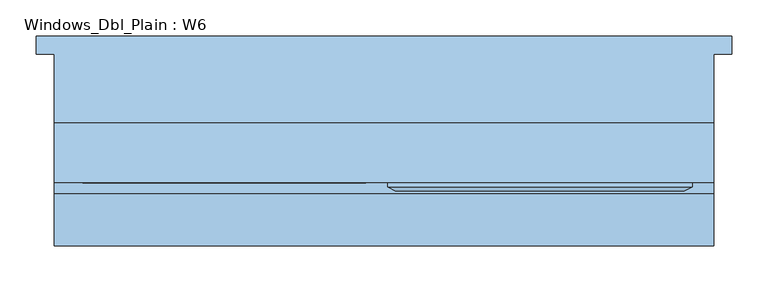
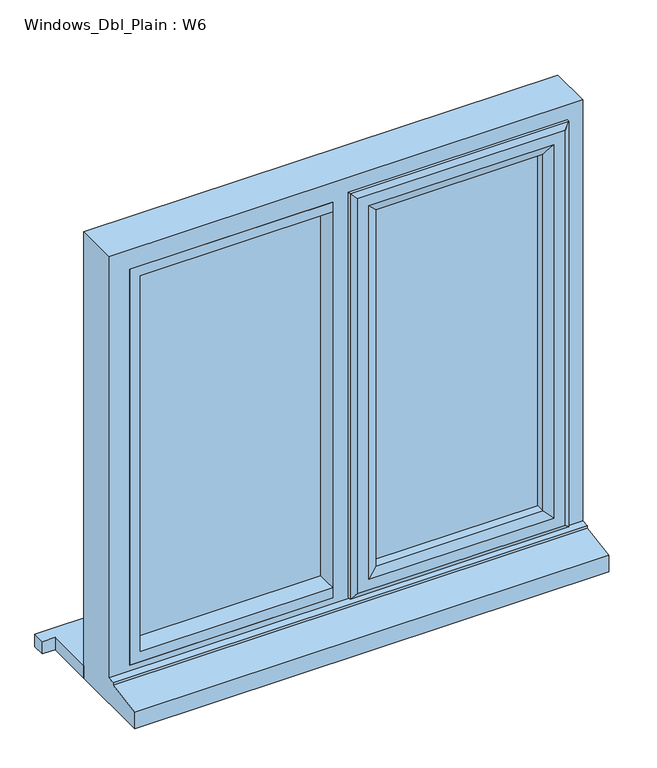
"""IFC4 building model written with IfcOpenShell, lengths in millimetres: window geometry, Windows_Dbl_Plain : W6."""

from ifc_helpers import new_model, si_unit, frame, origin, place, context, project, spatial, polyline, outline, extrude, faceted_brep, source, transform, mapped, element, save


def windows_dbl_plain_w6_14064f4c(model_context):
    return source(origin(), model_context, "Body", "SolidModel", [
        extrude(outline(polyline([(-767.2, 130.8434322), (197.2, 130.8434322), (197.2, 105.8434322), (172.2, 105.8434322), (172.2, 10.2434322), (-742.2, 10.2434322), (-742.2, 105.8434322), (-767.2, 105.8434322), (-767.2, 130.8434322)])), frame((0.0, 0.0, 1200.0), z_axis=(0.0, 0.0, 1.0), x_axis=(1.0, 0.0, 0.0)), (0.0, 0.0, 1.0), 25.0),
        faceted_brep([(-280.0, -72.7565678, 2080.0), (-280.0, -72.7565678, 1253.0), (-280.0, -78.5300705, 1253.0), (-280.0, -78.5300705, 2080.0), (-270.0, -7.7565678, 2070.0), (-270.0, -7.7565678, 1263.0), (-270.0, -72.7565678, 1263.0), (-270.0, -72.7565678, 2070.0), (-230.0, -22.2494677, 2030.0), (-230.0, -22.2494677, 1303.0), (-240.1480377, -7.7565678, 1292.8519623), (-240.1480377, -7.7565678, 2040.1480377), (-230.0, -36.7565678, 2030.0), (-230.0, -36.7565678, 1303.0), (-240.0, -60.7565678, 2040.0), (-240.0, -60.7565678, 1293.0), (-240.0, -36.7565678, 1293.0), (-240.0, -36.7565678, 2040.0), (-230.0, -78.5300705, 2030.0), (-230.0, -78.5300705, 1303.0), (-230.0, -60.7565678, 1303.0), (-230.0, -60.7565678, 2030.0), (-247.4457548, -84.3035732, 2047.4457548), (-247.4457548, -84.3035732, 1285.5542452), (-269.2153903, -84.3035732, 1263.7846097), (-269.2153903, -84.3035732, 2069.2153903), (142.2, -72.7565678, 1253.0), (142.2, -78.5300705, 1253.0), (132.2, -7.7565678, 1263.0), (132.2, -72.7565678, 1263.0), (92.2, -22.2494677, 1303.0), (102.3480377, -7.7565678, 1292.8519623), (92.2, -36.7565678, 1303.0), (102.2, -60.7565678, 1293.0), (102.2, -36.7565678, 1293.0), (92.2, -78.5300705, 1303.0), (92.2, -60.7565678, 1303.0), (109.6457548, -84.3035732, 1285.5542452), (131.4153903, -84.3035732, 1263.7846097), (142.2, -72.7565678, 2080.0), (142.2, -78.5300705, 2080.0), (132.2, -7.7565678, 2070.0), (132.2, -72.7565678, 2070.0), (92.2, -22.2494677, 2030.0), (102.3480377, -7.7565678, 2040.1480377), (92.2, -36.7565678, 2030.0), (102.2, -60.7565678, 2040.0), (102.2, -36.7565678, 2040.0), (92.2, -78.5300705, 2030.0), (92.2, -60.7565678, 2030.0), (109.6457548, -84.3035732, 2047.4457548), (131.4153903, -84.3035732, 2069.2153903)], [[[0, 1, 2, 3]], [[4, 5, 6, 7]], [[8, 9, 10, 11]], [[12, 13, 9, 8]], [[14, 15, 16, 17]], [[18, 19, 20, 21]], [[22, 23, 19, 18]], [[3, 2, 24, 25]], [[1, 26, 27, 2]], [[5, 28, 29, 6]], [[9, 30, 31, 10]], [[13, 32, 30, 9]], [[15, 33, 34, 16]], [[19, 35, 36, 20]], [[23, 37, 35, 19]], [[2, 27, 38, 24]], [[26, 39, 40, 27]], [[28, 41, 42, 29]], [[30, 43, 44, 31]], [[32, 45, 43, 30]], [[33, 46, 47, 34]], [[35, 48, 49, 36]], [[37, 50, 48, 35]], [[27, 40, 51, 38]], [[39, 0, 3, 40]], [[1, 0, 39, 26], [7, 6, 29, 42]], [[41, 4, 7, 42]], [[5, 4, 41, 28], [11, 10, 31, 44]], [[43, 8, 11, 44]], [[45, 12, 8, 43]], [[17, 16, 34, 47], [13, 12, 45, 32]], [[46, 14, 17, 47]], [[15, 14, 46, 33], [21, 20, 36, 49]], [[48, 18, 21, 49]], [[50, 22, 18, 48]], [[25, 24, 38, 51], [23, 22, 50, 37]], [[40, 3, 25, 51]]]),
        extrude(outline(polyline([(2070.0, -310.0), (2070.0, -702.2), (1263.0, -702.2), (1263.0, -310.0), (1283.0, -310.0), (1283.0, -682.2), (2050.0, -682.2), (2050.0, -310.0), (2070.0, -310.0)])), frame((0.0, -72.7565678, 0.0), z_axis=(0.0, 1.0, 0.0), x_axis=(0.0, 0.0, 1.0)), (0.0, 0.0, 1.0), 41.0),
        faceted_brep([(172.2, 10.2434322, 2110.0), (172.2, 10.2434322, 1200.0), (-742.2, 10.2434322, 1200.0), (-742.2, 10.2434322, 2110.0), (112.2, 10.2434322, 2050.0), (-252.0, 10.2434322, 2050.0), (-252.0, 10.2434322, 1275.0), (112.2, 10.2434322, 1275.0), (-310.0, 10.2434322, 2050.0), (-682.2, 10.2434322, 2050.0), (-682.2, 10.2434322, 1275.0), (-310.0, 10.2434322, 1275.0), (-742.2, -160.2565678, 1200.0), (-742.2, -160.2565678, 1233.8088847), (-742.2, -87.7565678, 1244.7449676), (-742.2, -87.7565678, 1249.68767), (-742.2, -72.7565678, 1251.0), (-742.2, -72.7565678, 2110.0), (172.2, -72.7565678, 1251.0), (172.2, -72.7565678, 2110.0), (-702.2, -72.7565678, 2070.0), (-310.0, -72.7565678, 2070.0), (-310.0, -72.7565678, 1263.0), (-702.2, -72.7565678, 1263.0), (-270.0, -72.7565678, 2070.0), (132.2, -72.7565678, 2070.0), (132.2, -72.7565678, 1263.0), (-270.0, -72.7565678, 1263.0), (-702.2, -7.7565678, 1263.0), (-702.2, -7.7565678, 2070.0), (-300.0, -7.7565678, 1263.0), (-300.0, -7.7565678, 2070.0), (-310.0, -7.7565678, 2050.0), (-310.0, -7.7565678, 1275.0), (-682.2, -7.7565678, 1275.0), (-682.2, -7.7565678, 2050.0), (-270.0, -7.7565678, 2070.0), (-270.0, -7.7565678, 1263.0), (132.2, -7.7565678, 1263.0), (132.2, -7.7565678, 2070.0), (112.2, -7.7565678, 2050.0), (112.2, -7.7565678, 1275.0), (-252.0, -7.7565678, 1275.0), (-252.0, -7.7565678, 2050.0), (-300.0, -31.7565678, 2070.0), (-310.0, -31.7565678, 2070.0), (172.2, -87.7565678, 1249.68767), (172.2, -87.7565678, 1244.7449676), (172.2, -160.2565678, 1233.8088847), (172.2, -160.2565678, 1200.0), (-300.0, -31.7565678, 1263.0), (-310.0, -31.7565678, 1263.0)], [[[0, 1, 2, 3], [4, 5, 6, 7], [8, 9, 10, 11]], [[2, 12, 13, 14, 15, 16, 17, 3]], [[16, 18, 19, 17], [20, 21, 22, 23], [24, 25, 26, 27]], [[23, 28, 29, 20]], [[29, 28, 30, 31], [32, 33, 34, 35]], [[36, 37, 38, 39], [40, 41, 42, 43]], [[35, 34, 10, 9]], [[3, 17, 19, 0]], [[25, 24, 36, 39]], [[29, 31, 44, 45, 21, 20]], [[9, 8, 32, 35]], [[40, 43, 5, 4]], [[18, 46, 47, 48, 49, 1, 0, 19]], [[25, 39, 38, 26]], [[4, 7, 41, 40]], [[44, 31, 30, 50]], [[50, 51, 45, 44]], [[51, 22, 21, 45]], [[27, 37, 36, 24]], [[43, 42, 6, 5]], [[8, 11, 33, 32]], [[49, 12, 2, 1]], [[48, 13, 12, 49]], [[47, 14, 13, 48]], [[46, 15, 14, 47]], [[18, 16, 15, 46]], [[26, 38, 37, 27]], [[22, 51, 50, 30, 28, 23]], [[6, 42, 41, 7]], [[33, 11, 10, 34]]]),
        extrude(outline(polyline([(-702.2, -31.7565678), (-702.2, -7.7565678), (-300.0, -7.7565678), (-300.0, -31.7565678), (-702.2, -31.7565678)])), frame((0.0, 0.0, 1263.0), z_axis=(0.0, 0.0, 1.0), x_axis=(1.0, 0.0, 0.0)), (0.0, 0.0, 1.0), 807.0),
        extrude(outline(polyline([(102.2, -36.7565678), (102.2, -60.7565678), (-240.0, -60.7565678), (-240.0, -36.7565678), (102.2, -36.7565678)])), frame((0.0, 0.0, 1293.0), z_axis=(0.0, 0.0, 1.0), x_axis=(1.0, 0.0, 0.0)), (0.0, 0.0, 1.0), 747.0),
    ])


if __name__ == "__main__":
    model = new_model("IFC4")
    model_context = context("Model", 3, world=origin())
    ifc_project = project(units=[si_unit("LENGTHUNIT", "METRE", prefix="MILLI")], contexts=[model_context])
    site = spatial("IfcSite", under=ifc_project)
    building = spatial("IfcBuilding", under=site)
    placement = place(None, origin())
    windows_dbl_plain_w6_shape = windows_dbl_plain_w6_14064f4c(model_context)
    element("IfcWindow", 1, ObjectType="Windows_Dbl_Plain : W6", at=placement, inside=building, context=model_context, shape_type="MappedRepresentation", body=[
        mapped(windows_dbl_plain_w6_shape, transform((0.0, 0.0, 0.0), x_axis=(1.0, 0.0, 0.0), y_axis=(0.0, 1.0, 0.0), z_axis=(0.0, 0.0, 1.0))),
    ])
    save(model, "model.ifc")

# Revit data of these elements
# Type "Windows_Dbl_Plain : W6"
#   Type Mark = "56"
#   Operation = "DoublePanelVertical"
#   Construction Type Id = "GSP4R"
#   Manufacturer = "Revit"
#   Keynote = "L10"
#   Analytic Construction = "1/8 in Pilkington single glazing"
#   Wrap Layers (Ext) from Ext = 0.336286 ft
#   Wrap Layers (Int) from Ext = 0.582349 ft
#   Window Board Projection = 0.082021 ft
#   Window Board Extension = 0.082021 ft
#   Visual Light Transmittance = 0.9
#   Solar Heat Gain Coefficient = 0.78
#   Rough Width = 3.0 ft
#   Rough Height = 2.985564 ft
#   Height = 2.985564 ft
#   Width = 3.0 ft
#   Heat Transfer Coefficient (U) = 3.6886 W/(m²·K)
#   Glazing Thickness = 0.07874 ft
#   FrameOffset - External = 0.164042 ft
#   Frame Depth = 0.213255 ft
#   Default Head Height = 6.922572 ft
#   Cill Depth = 0.287073 ft
#   Cavity Closer Width = 0.164042 ft
#   Cavity Closer Offset from Ext = 0.336286 ft
#   Cavity Closer Depth = 0.278871 ft
#   Vis - Cavity Closers = yes
#   Define Thermal Properties by = 1
#   Material Trim = Window Frame
#   Material Glass = Glass
#   Material Frame = Cherry
#   Wall Closure = (empty or 0)
# Element 1 (IfcWindow, "Windows_Dbl_Plain : W6")
#   Materials on its faces: "Cherry", "Glass", "Window Frame"
# Materials
#   "Window Frame": colour RGB 249 249 249, transparency 0, Keynote = "L10", Cost = 0
#   "Glass": class "Glass", colour RGB 0 128 192, transparency 0.9, Description = "Soda Lime Glass", Cost = 0
#   "Cherry": class "Wood", colour RGB 226 177 128, transparency 0, Description = "Prunus Serotina", Cost = 0
